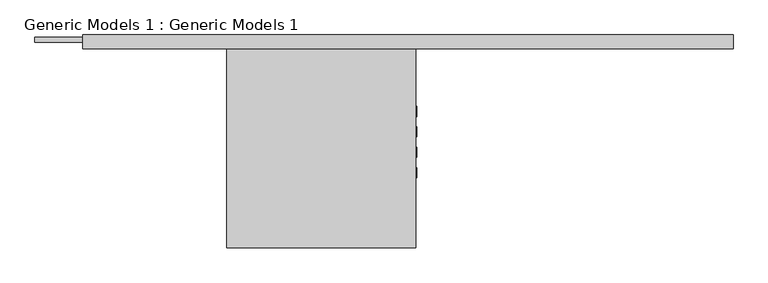
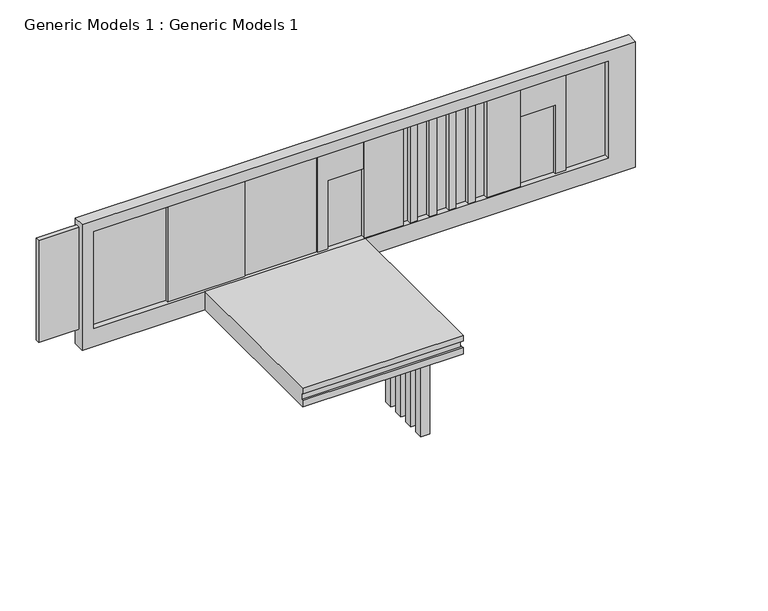
"""IFC4 building model written with IfcOpenShell, lengths in millimetres: proxy geometry, Generic Models 1 : Generic Models 1."""

from ifc_helpers import new_model, si_unit, frame, origin, origin_with_axes, place, context, project, spatial, polyline, outline, extrude, faceted_brep, source, transform, mapped, element, save


def generic_models_1_generic_models_1_486b888d(model_context):
    return source(origin(), model_context, "Body", "SolidModel", [
        faceted_brep([(-4975.9237038, -15354.9479847, 3200.4), (-750.1431282, -15354.9479847, 3200.4), (-750.1431282, -15354.9479847, 3378.2), (-4975.9237038, -15354.9479847, 3378.2), (-750.1431282, -15354.9479847, 3708.4), (-4975.9237038, -15354.9479847, 3708.4), (-4975.9237038, -15354.9479847, 3552.4232929), (-750.1431282, -15354.9479847, 3552.4232929), (-4975.9237038, -10890.6779557, 3708.4), (-750.1431282, -10890.6779557, 3708.4), (-750.1431282, -10890.6779557, 3552.4232929), (-800.9431282, -10890.6779557, 3552.4232929), (-800.9431282, -10890.6779557, 3374.6232929), (-750.1431282, -10890.6779557, 3374.6232929), (-750.1431282, -10890.6779557, 3200.4), (-4975.9237038, -10890.6779557, 3200.4), (-4975.9237038, -15304.1479847, 3378.2), (-4975.9237038, -15304.1479847, 3552.4232929), (-750.1431282, -15304.1479847, 3374.6232929), (-750.1431282, -15304.1479847, 3378.2), (-800.9431282, -15304.1479847, 3378.2), (-800.9431282, -15304.1479847, 3552.4232929), (-800.9431282, -15304.1479847, 3374.6232929)], [[[0, 1, 2, 3]], [[4, 5, 6, 7]], [[8, 9, 10, 11, 12, 13, 14, 15]], [[8, 15, 0, 3, 16, 17, 6, 5]], [[1, 0, 15, 14]], [[1, 14, 13, 18, 19, 2]], [[9, 4, 7, 10]], [[5, 4, 9, 8]], [[17, 16, 20, 21]], [[7, 6, 17, 21, 11, 10]], [[3, 2, 19, 20, 16]], [[22, 12, 11, 21, 20]], [[18, 22, 20, 19]], [[12, 22, 18, 13]]]),
        extrude(outline(polyline([(-953.3431282, -12186.0779557), (-724.7431282, -12186.0779557), (-724.7431282, -12414.6779557), (-953.3431282, -12414.6779557), (-953.3431282, -12186.0779557)])), origin_with_axes(), (0.0, 0.0, 1.0), 3200.4),
        extrude(outline(polyline([(-953.3431282, -12643.2779557), (-724.7431282, -12643.2779557), (-724.7431282, -12871.8779557), (-953.3431282, -12871.8779557), (-953.3431282, -12643.2779557)])), origin_with_axes(), (0.0, 0.0, 1.0), 3200.4),
        extrude(outline(polyline([(-953.3431282, -13100.4779557), (-724.7431282, -13100.4779557), (-724.7431282, -13329.0779557), (-953.3431282, -13329.0779557), (-953.3431282, -13100.4779557)])), origin_with_axes(), (0.0, 0.0, 1.0), 3200.4),
        extrude(outline(polyline([(-953.3431282, -13557.6779557), (-724.7431282, -13557.6779557), (-724.7431282, -13786.2779557), (-953.3431282, -13786.2779557), (-953.3431282, -13557.6779557)])), origin_with_axes(), (0.0, 0.0, 1.0), 3200.4),
        extrude(outline(polyline([(-3892.8441472, -10827.1779557), (-5918.7637858, -10827.1779557), (-5918.7637858, -10750.9779557), (-3892.8441472, -10750.9779557), (-3892.8441472, -10827.1779557)])), frame((0.0, 0.0, 3708.4), z_axis=(0.0, 0.0, 1.0), x_axis=(1.0, 0.0, 0.0)), (0.0, 0.0, 1.0), 2692.4),
        extrude(outline(polyline([(-1978.1947325, -10801.7779557), (-3892.8441472, -10801.7779557), (-3892.8441472, -10750.9779557), (-1978.1947325, -10750.9779557), (-1978.1947325, -10801.7779557)])), frame((0.0, 0.0, 3708.4), z_axis=(0.0, 0.0, 1.0), x_axis=(1.0, 0.0, 0.0)), (0.0, 0.0, 1.0), 2692.4),
        extrude(outline(polyline([(3708.4, -1698.7947325), (5613.4, -1698.7947325), (5613.4, -758.9947325), (6400.8, -758.9947325), (6400.8, -1978.1947325), (3708.4, -1978.1947325), (3708.4, -1698.7947325)])), frame((0.0, -10827.1779557, 0.0), z_axis=(0.0, 1.0, 0.0), x_axis=(0.0, 0.0, 1.0)), (0.0, 0.0, 1.0), 76.2),
        extrude(outline(polyline([(-762.8431282, -10750.9779557), (260.5535042, -10750.9779557), (260.5535042, -10877.9779557), (-762.8431282, -10877.9779557), (-762.8431282, -10750.9779557)])), frame((0.0, 0.0, 3708.4), z_axis=(0.0, 0.0, 1.0), x_axis=(1.0, 0.0, 0.0)), (0.0, 0.0, 1.0), 2692.4),
        extrude(outline(polyline([(440.3999112, -10750.9779557), (630.3537838, -10750.9779557), (630.3537838, -10877.9779557), (440.3999112, -10877.9779557), (440.3999112, -10750.9779557)])), frame((0.0, 0.0, 3708.4), z_axis=(0.0, 0.0, 1.0), x_axis=(1.0, 0.0, 0.0)), (0.0, 0.0, 1.0), 2692.4),
        extrude(outline(polyline([(948.3999112, -10750.9779557), (1138.3537838, -10750.9779557), (1138.3537838, -10877.9779557), (948.3999112, -10877.9779557), (948.3999112, -10750.9779557)])), frame((0.0, 0.0, 3708.4), z_axis=(0.0, 0.0, 1.0), x_axis=(1.0, 0.0, 0.0)), (0.0, 0.0, 1.0), 2692.4),
        extrude(outline(polyline([(1456.3999112, -10750.9779557), (1646.3537838, -10750.9779557), (1646.3537838, -10877.9779557), (1456.3999112, -10877.9779557), (1456.3999112, -10750.9779557)])), frame((0.0, 0.0, 3708.4), z_axis=(0.0, 0.0, 1.0), x_axis=(1.0, 0.0, 0.0)), (0.0, 0.0, 1.0), 2692.4),
        extrude(outline(polyline([(1970.7499112, -10750.9779557), (2160.7037838, -10750.9779557), (2160.7037838, -10877.9779557), (1970.7499112, -10877.9779557), (1970.7499112, -10750.9779557)])), frame((0.0, 0.0, 3708.4), z_axis=(0.0, 0.0, 1.0), x_axis=(1.0, 0.0, 0.0)), (0.0, 0.0, 1.0), 2692.4),
        extrude(outline(polyline([(3335.9999112, -10877.9779557), (2455.9787838, -10877.9779557), (2455.9787838, -10750.9779557), (3335.9999112, -10750.9779557), (3335.9999112, -10877.9779557)])), frame((0.0, 0.0, 3708.4), z_axis=(0.0, 0.0, 1.0), x_axis=(1.0, 0.0, 0.0)), (0.0, 0.0, 1.0), 2692.4),
        extrude(outline(polyline([(3708.4, 4287.9084761), (3708.4, 4567.3084761), (6400.8, 4567.3084761), (6400.8, 3348.1084761), (5613.4, 3348.1084761), (5613.4, 4287.9084761), (3708.4, 4287.9084761)])), frame((0.0, -10827.1779557, 0.0), z_axis=(0.0, 1.0, 0.0), x_axis=(0.0, 0.0, 1.0)), (0.0, 0.0, 1.0), 76.2),
        extrude(outline(polyline([(-9276.4435762, -10643.0279557), (5651.3208786, -10643.0279557), (5651.3208786, -10750.9779557), (-9276.4435762, -10750.9779557), (-9276.4435762, -10643.0279557)])), frame((0.0, 0.0, 3708.4), z_axis=(0.0, 0.0, 1.0), x_axis=(1.0, 0.0, 0.0)), (0.0, 0.0, 1.0), 2844.8),
        extrude(outline(polyline([(6705.6, 6362.5208786), (6705.6, -8210.307583), (3200.4, -8210.307583), (3200.4, 6362.5208786), (6705.6, 6362.5208786)]), holes=[polyline([(3708.4, -7905.507583), (6400.8, -7905.507583), (6400.8, 5651.3208786), (3708.4, 5651.3208786), (3708.4, -7905.507583)])]), frame((0.0, -10890.6779557, 0.0), z_axis=(0.0, 1.0, 0.0), x_axis=(0.0, 0.0, 1.0)), (0.0, 0.0, 1.0), 304.8),
    ])


if __name__ == "__main__":
    model = new_model("IFC4")
    model_context = context("Model", 3, world=origin())
    ifc_project = project(units=[si_unit("LENGTHUNIT", "METRE", prefix="MILLI")], contexts=[model_context])
    site = spatial("IfcSite", under=ifc_project)
    building = spatial("IfcBuilding", under=site)
    placement = place(None, origin())
    generic_models_1_generic_models_1_shape = generic_models_1_generic_models_1_486b888d(model_context)
    element("IfcBuildingElementProxy", 1, Name="Generic Models 1 : Generic Models 1", ObjectType="Generic Models 1 : Generic Models 1", at=placement, inside=building, context=model_context, shape_type="MappedRepresentation", body=[
        mapped(generic_models_1_generic_models_1_shape, transform((0.0, 0.0, 0.0), x_axis=(1.0, 0.0, 0.0), y_axis=(0.0, 1.0, 0.0), z_axis=(0.0, 0.0, 1.0))),
    ])
    save(model, "model.ifc")

# Revit data of these elements
# Element 1 (IfcBuildingElementProxy, "Generic Models 1 : Generic Models 1")
#   Materials on its faces: "Gypsum Wall Board", "wood", "Water"
# Materials
#   "Gypsum Wall Board": class "Generic", colour RGB 127 127 127, transparency 0, Description = "Gypsum Wall Board", Cost = 0
#   "wood": class "Generic", colour RGB 120 120 120, transparency 0, Cost = 0
#   "Water": class "Liquid", colour RGB 108 195 217, transparency 0.7, Description = "Water", Cost = 0
